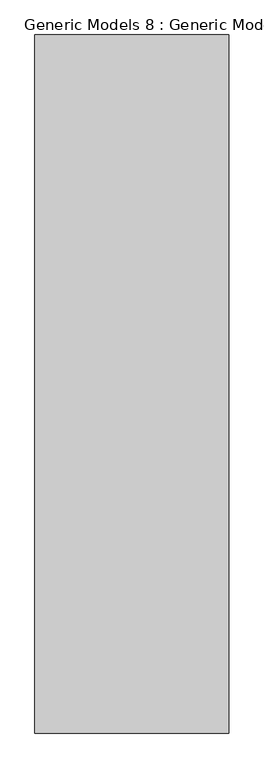
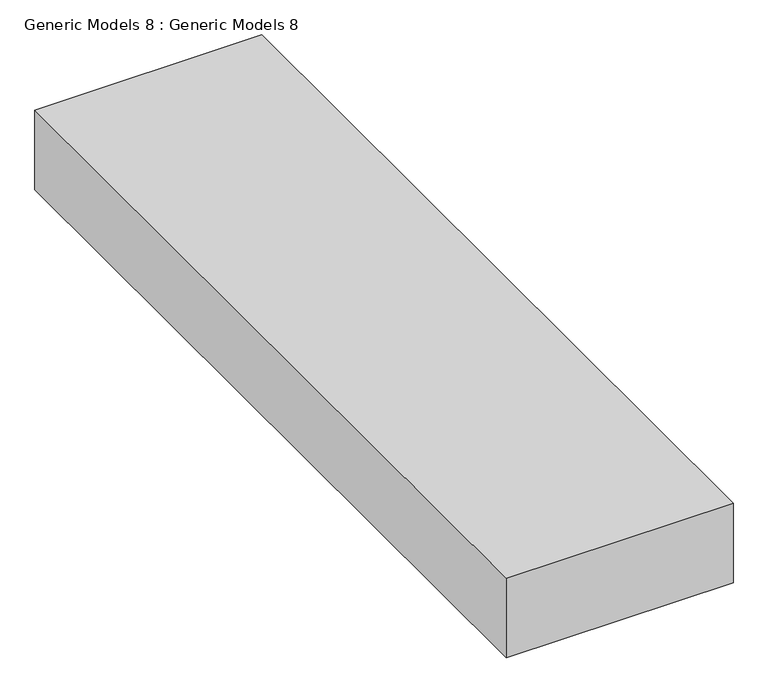
"""IFC4 building model written with IfcOpenShell, lengths in millimetres: proxy geometry, Generic Models 8 : Generic Models 8."""

from ifc_helpers import new_model, si_unit, frame, origin, place, context, project, spatial, polyline, outline, extrude, source, transform, mapped, element, save


def generic_models_8_generic_models_8_3ed65b9d(model_context):
    return source(origin(), model_context, "Body", "SweptSolid", [
        extrude(outline(polyline([(-3391.6221861, 3019.8222768), (-3391.6221861, 1541.4927862), (-3802.4859258, 1541.4927862), (-3802.4859258, 3019.8222768), (-3391.6221861, 3019.8222768)])), frame((0.0, 0.0, 2473.010234), z_axis=(0.0, 0.0, 1.0), x_axis=(1.0, 0.0, 0.0)), (0.0, 0.0, 1.0), 152.4),
    ])


if __name__ == "__main__":
    model = new_model("IFC4")
    model_context = context("Model", 3, world=origin())
    ifc_project = project(units=[si_unit("LENGTHUNIT", "METRE", prefix="MILLI")], contexts=[model_context])
    site = spatial("IfcSite", under=ifc_project)
    building = spatial("IfcBuilding", under=site)
    placement = place(None, origin())
    generic_models_8_generic_models_8_shape = generic_models_8_generic_models_8_3ed65b9d(model_context)
    element("IfcBuildingElementProxy", 1, Name="Generic Models 8 : Generic Models 8", ObjectType="Generic Models 8 : Generic Models 8", at=placement, inside=building, context=model_context, shape_type="MappedRepresentation", body=[
        mapped(generic_models_8_generic_models_8_shape, transform((0.0, 0.0, 0.0), x_axis=(1.0, 0.0, 0.0), y_axis=(0.0, 1.0, 0.0), z_axis=(0.0, 0.0, 1.0))),
    ])
    save(model, "model.ifc")
